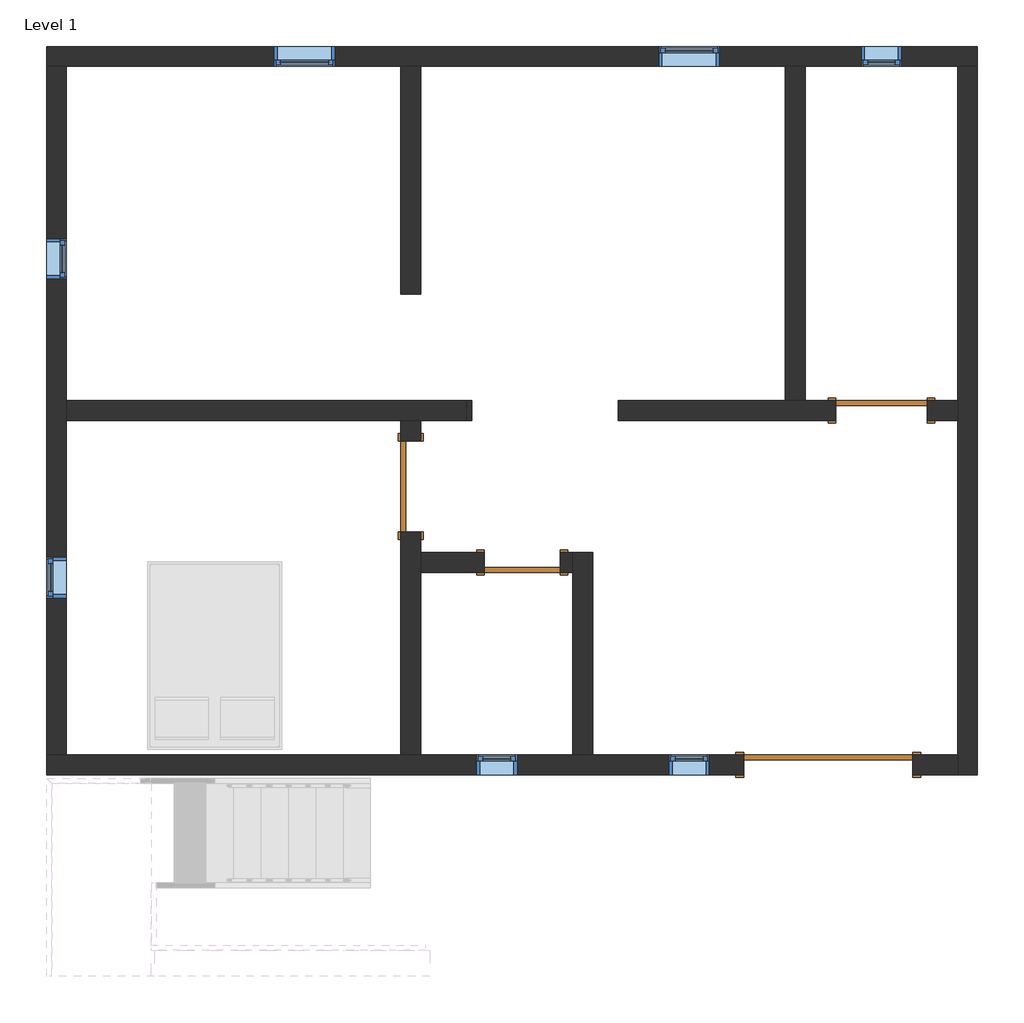
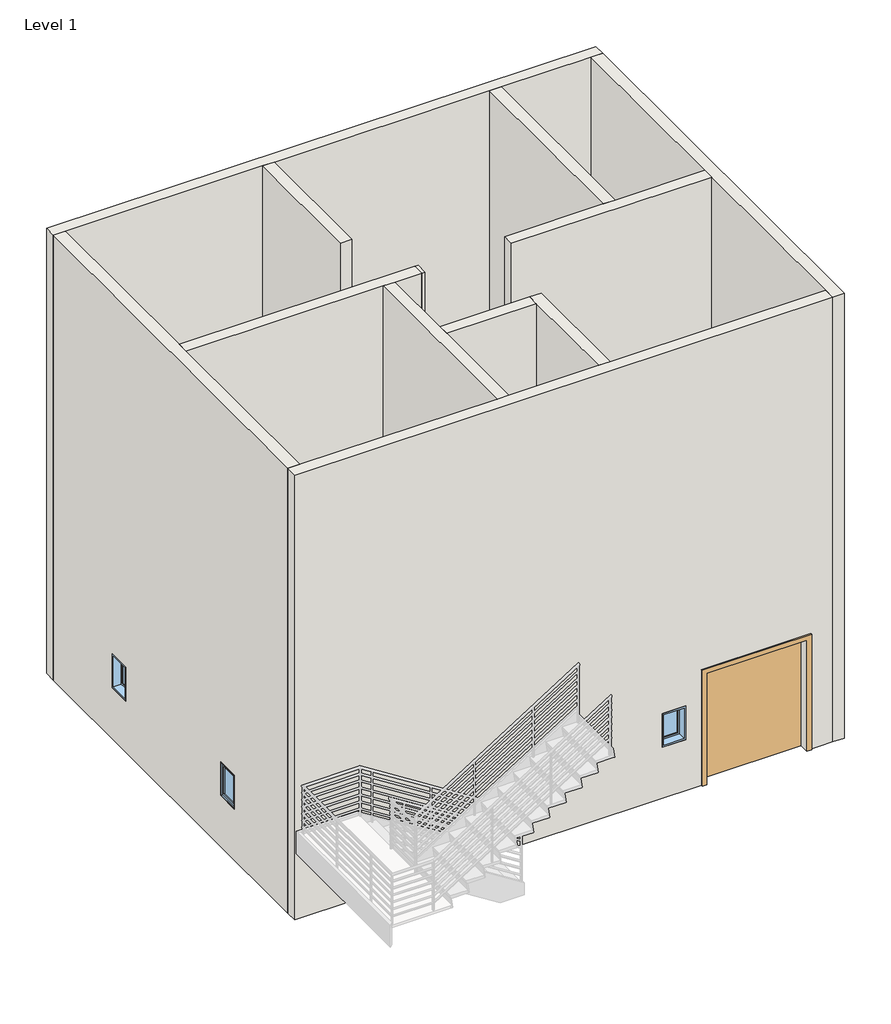
# One storey, part 1 of 4: 12 walls, 7 windows, 4 doors.
"""IFC4 building model written with IfcOpenShell, lengths in millimetres."""

from ifc_helpers import new_model, si_unit, frame, origin, origin_with_axes, place, context, project, spatial, polyline, outline, extrude, faceted_brep, transform, mapped, element, save
from components import m_door_double_flush_panel_double_acting_1700_x_2000mm_0a6d9c7f, m_single_flush_0762_x_2032mm_7341a4fb, m_single_flush_0915_x_2134mm_6a9e8738, m_fixed_0406_x_0610mm_8205b201, m_fixed_0610_x_1220mm_4e981104

model = new_model("IFC4")

# Units and contexts
model_context = context("Model", 3, world=origin())
ifc_project = project(units=[si_unit("LENGTHUNIT", "METRE", prefix="MILLI")], contexts=[model_context])

# Site, building, storey
site = spatial("IfcSite", under=ifc_project)
building = spatial("IfcBuilding", under=site)
storey = spatial("IfcBuildingStorey", under=building, Name="Level 1", Elevation=0.0)

# Doors
placement = place(None, origin())
m_door_double_flush_panel_double_acting_1700_x_2000mm_shape = m_door_double_flush_panel_double_acting_1700_x_2000mm_0a6d9c7f(model_context)
element("IfcDoor", 1, ObjectType="M_Door-Double-Flush_Panel-Double-Acting : 1700 x 2000mm", at=placement, inside=storey, context=model_context, shape_type="MappedRepresentation", body=[
    mapped(m_door_double_flush_panel_double_acting_1700_x_2000mm_shape, transform((-3679.0492596, 6432.7433377, 0.0), x_axis=(1.0, 0.0, 0.0), y_axis=(0.0, 1.0, 0.0), z_axis=(0.0, 0.0, 1.0))),
])
m_single_flush_0762_x_2032mm_shape = m_single_flush_0762_x_2032mm_7341a4fb(model_context)
element("IfcDoor", 2, ObjectType="M_Single-Flush : 0762 x 2032mm", at=placement, inside=storey, context=model_context, shape_type="MappedRepresentation", body=[
    mapped(m_single_flush_0762_x_2032mm_shape, transform((-6752.4492596, 8463.1433377, 0.0), x_axis=(1.0, 0.0, 0.0), y_axis=(0.0, 1.0, 0.0), z_axis=(0.0, 0.0, 1.0))),
])
m_single_flush_0915_x_2134mm_shape = m_single_flush_0915_x_2134mm_6a9e8738(model_context)
element("IfcDoor", 3, ObjectType="M_Single-Flush : 0915 x 2134mm", at=placement, inside=storey, context=model_context, shape_type="MappedRepresentation", body=[
    mapped(m_single_flush_0915_x_2134mm_shape, transform((-3145.6492596, 9988.7433377, 0.0), x_axis=(1.0, 0.0, 0.0), y_axis=(0.0, 1.0, 0.0), z_axis=(0.0, 0.0, 1.0))),
])
element("IfcDoor", 4, ObjectType="M_Single-Flush : 0915 x 2134mm", at=placement, inside=storey, context=model_context, shape_type="MappedRepresentation", body=[
    mapped(m_single_flush_0915_x_2134mm_shape, transform((-7870.0492596, 9226.7433377, 0.0), x_axis=(0.0, 1.0, 0.0), y_axis=(-1.0, 0.0, 0.0), z_axis=(0.0, 0.0, 1.0))),
])

# Walls
element("IfcWall", 5, ObjectType="Generic - 200mm", at=placement, inside=storey, context=model_context, shape_type="Brep", body=[
    faceted_brep([(-11526.0492596, 13444.7433377, 0.0), (-11326.0492596, 13444.7433377, 0.0), (-7970.0492596, 13444.7433377, 0.0), (-7770.0492596, 13444.7433377, 0.0), (-4109.2492596, 13444.7433377, 0.0), (-3909.2492596, 13444.7433377, 0.0), (-2382.0492596, 13444.7433377, 0.0), (-2182.0492596, 13444.7433377, 0.0), (-2182.0492596, 13444.7433377, 8000.0), (-2382.0492596, 13444.7433377, 8000.0), (-3909.2492596, 13444.7433377, 8000.0), (-4109.2492596, 13444.7433377, 8000.0), (-7770.0492596, 13444.7433377, 8000.0), (-7970.0492596, 13444.7433377, 8000.0), (-11326.0492596, 13444.7433377, 8000.0), (-11526.0492596, 13444.7433377, 8000.0), (-8631.8492596, 13444.7433377, 915.0), (-9241.8492596, 13444.7433377, 915.0), (-9241.8492596, 13444.7433377, 2135.0), (-8631.8492596, 13444.7433377, 2135.0), (-5381.0492596, 13444.7433377, 915.0), (-5381.0492596, 13444.7433377, 2135.0), (-4771.0492596, 13444.7433377, 2135.0), (-4771.0492596, 13444.7433377, 915.0), (-2942.6492596, 13444.7433377, 915.0), (-3348.6492596, 13444.7433377, 915.0), (-3348.6492596, 13444.7433377, 1525.0), (-2942.6492596, 13444.7433377, 1525.0), (-11526.0492596, 13644.7433377, 0.0), (-11526.0492596, 13644.7433377, 8000.0), (-2182.0492596, 13644.7433377, 8000.0), (-2182.0492596, 13644.7433377, 0.0), (-8631.8492596, 13644.7433377, 915.0), (-8631.8492596, 13644.7433377, 2135.0), (-9241.8492596, 13644.7433377, 2135.0), (-9241.8492596, 13644.7433377, 915.0), (-5381.0492596, 13644.7433377, 915.0), (-4771.0492596, 13644.7433377, 915.0), (-4771.0492596, 13644.7433377, 2135.0), (-5381.0492596, 13644.7433377, 2135.0), (-2942.6492596, 13644.7433377, 915.0), (-2942.6492596, 13644.7433377, 1525.0), (-3348.6492596, 13644.7433377, 1525.0), (-3348.6492596, 13644.7433377, 915.0)], [[[0, 1, 2, 3, 4, 5, 6, 7, 8, 9, 10, 11, 12, 13, 14, 15], [16, 17, 18, 19], [20, 21, 22, 23], [24, 25, 26, 27]], [[28, 29, 30, 31], [32, 33, 34, 35], [36, 37, 38, 39], [40, 41, 42, 43]], [[7, 6, 5, 4, 3, 2, 1, 0, 28, 31]], [[15, 14, 13, 12, 11, 10, 9, 8, 30, 29]], [[8, 7, 31, 30]], [[0, 15, 29, 28]], [[33, 32, 16, 19]], [[34, 33, 19, 18]], [[35, 34, 18, 17]], [[32, 35, 17, 16]], [[21, 20, 36, 39]], [[22, 21, 39, 38]], [[23, 22, 38, 37]], [[20, 23, 37, 36]], [[41, 40, 24, 27]], [[42, 41, 27, 26]], [[43, 42, 26, 25]], [[40, 43, 25, 24]]]),
])
element("IfcWall", 6, ObjectType="Generic - 200mm", at=placement, inside=storey, context=model_context, shape_type="Brep", body=[
    faceted_brep([(-2382.0492596, 13444.7433377, 0.0), (-2382.0492596, 10088.7433377, 0.0), (-2382.0492596, 9888.7433377, 0.0), (-2382.0492596, 6532.7433377, 0.0), (-2382.0492596, 6332.7433377, 0.0), (-2382.0492596, 6332.7433377, 8000.0), (-2382.0492596, 6532.7433377, 8000.0), (-2382.0492596, 9888.7433377, 8000.0), (-2382.0492596, 10088.7433377, 8000.0), (-2382.0492596, 13444.7433377, 8000.0), (-2182.0492596, 13444.7433377, 0.0), (-2182.0492596, 13444.7433377, 8000.0), (-2182.0492596, 6332.7433377, 8000.0), (-2182.0492596, 6332.7433377, 0.0)], [[[0, 1, 2, 3, 4, 5, 6, 7, 8, 9]], [[10, 11, 12, 13]], [[4, 3, 2, 1, 0, 10, 13]], [[9, 8, 7, 6, 5, 12, 11]], [[0, 9, 11, 10]], [[5, 4, 13, 12]]]),
])
element("IfcWall", 7, ObjectType="Generic - 200mm", at=placement, inside=storey, context=model_context, shape_type="Brep", body=[
    faceted_brep([(-11526.0492596, 6532.7433377, 8000.0), (-11326.0492596, 6532.7433377, 8000.0), (-7970.0492596, 6532.7433377, 8000.0), (-7770.0492596, 6532.7433377, 8000.0), (-6242.8492596, 6532.7433377, 8000.0), (-6042.8492596, 6532.7433377, 8000.0), (-2382.0492596, 6532.7433377, 8000.0), (-2382.0492596, 6532.7433377, 0.0), (-2829.0492596, 6532.7433377, 0.0), (-2829.0492596, 6532.7433377, 2000.0), (-4529.0492596, 6532.7433377, 2000.0), (-4529.0492596, 6532.7433377, 0.0), (-6042.8492596, 6532.7433377, 0.0), (-6242.8492596, 6532.7433377, 0.0), (-7770.0492596, 6532.7433377, 0.0), (-7970.0492596, 6532.7433377, 0.0), (-11326.0492596, 6532.7433377, 0.0), (-11526.0492596, 6532.7433377, 0.0), (-7209.4492596, 6532.7433377, 915.0), (-6803.4492596, 6532.7433377, 915.0), (-6803.4492596, 6532.7433377, 1525.0), (-7209.4492596, 6532.7433377, 1525.0), (-5279.0492596, 6532.7433377, 915.0), (-4873.0492596, 6532.7433377, 915.0), (-4873.0492596, 6532.7433377, 1525.0), (-5279.0492596, 6532.7433377, 1525.0), (-2382.0492596, 6332.7433377, 8000.0), (-11526.0492596, 6332.7433377, 8000.0), (-11526.0492596, 6332.7433377, 0.0), (-4529.0492596, 6332.7433377, 0.0), (-4529.0492596, 6332.7433377, 2000.0), (-2829.0492596, 6332.7433377, 2000.0), (-2829.0492596, 6332.7433377, 0.0), (-2382.0492596, 6332.7433377, 0.0), (-7209.4492596, 6332.7433377, 915.0), (-7209.4492596, 6332.7433377, 1525.0), (-6803.4492596, 6332.7433377, 1525.0), (-6803.4492596, 6332.7433377, 915.0), (-5279.0492596, 6332.7433377, 915.0), (-5279.0492596, 6332.7433377, 1525.0), (-4873.0492596, 6332.7433377, 1525.0), (-4873.0492596, 6332.7433377, 915.0)], [[[0, 1, 2, 3, 4, 5, 6, 7, 8, 9, 10, 11, 12, 13, 14, 15, 16, 17], [18, 19, 20, 21], [22, 23, 24, 25]], [[26, 27, 28, 29, 30, 31, 32, 33], [34, 35, 36, 37], [38, 39, 40, 41]], [[7, 33, 32, 8]], [[28, 17, 16, 15, 14, 13, 12, 11, 29]], [[6, 5, 4, 3, 2, 1, 0, 27, 26]], [[7, 6, 26, 33]], [[0, 17, 28, 27]], [[35, 34, 18, 21]], [[36, 35, 21, 20]], [[37, 36, 20, 19]], [[34, 37, 19, 18]], [[39, 38, 22, 25]], [[40, 39, 25, 24]], [[41, 40, 24, 23]], [[38, 41, 23, 22]], [[31, 9, 8, 32]], [[9, 31, 30, 10]], [[10, 30, 29, 11]]]),
])
element("IfcWall", 8, ObjectType="Generic - 200mm", at=placement, inside=storey, context=model_context, shape_type="Brep", body=[
    faceted_brep([(-11326.0492596, 6532.7433377, 0.0), (-11326.0492596, 9888.7433377, 0.0), (-11326.0492596, 10088.7433377, 0.0), (-11326.0492596, 13444.7433377, 0.0), (-11326.0492596, 13444.7433377, 8000.0), (-11326.0492596, 10088.7433377, 8000.0), (-11326.0492596, 9888.7433377, 8000.0), (-11326.0492596, 6532.7433377, 8000.0), (-11326.0492596, 11715.7433377, 915.0), (-11326.0492596, 11309.7433377, 915.0), (-11326.0492596, 11309.7433377, 1525.0), (-11326.0492596, 11715.7433377, 1525.0), (-11326.0492596, 8109.3433377, 915.0), (-11326.0492596, 8109.3433377, 1525.0), (-11326.0492596, 8515.3433377, 1525.0), (-11326.0492596, 8515.3433377, 915.0), (-11526.0492596, 6532.7433377, 0.0), (-11526.0492596, 6532.7433377, 8000.0), (-11526.0492596, 13444.7433377, 8000.0), (-11526.0492596, 13444.7433377, 0.0), (-11526.0492596, 11715.7433377, 915.0), (-11526.0492596, 11715.7433377, 1525.0), (-11526.0492596, 11309.7433377, 1525.0), (-11526.0492596, 11309.7433377, 915.0), (-11526.0492596, 8109.3433377, 915.0), (-11526.0492596, 8515.3433377, 915.0), (-11526.0492596, 8515.3433377, 1525.0), (-11526.0492596, 8109.3433377, 1525.0)], [[[0, 1, 2, 3, 4, 5, 6, 7], [8, 9, 10, 11], [12, 13, 14, 15]], [[16, 17, 18, 19], [20, 21, 22, 23], [24, 25, 26, 27]], [[3, 2, 1, 0, 16, 19]], [[7, 6, 5, 4, 18, 17]], [[4, 3, 19, 18]], [[0, 7, 17, 16]], [[21, 20, 8, 11]], [[22, 21, 11, 10]], [[23, 22, 10, 9]], [[20, 23, 9, 8]], [[13, 12, 24, 27]], [[14, 13, 27, 26]], [[15, 14, 26, 25]], [[12, 15, 25, 24]]]),
])
element("IfcWall", 9, ObjectType="Generic - 200mm", at=placement, inside=storey, context=model_context, shape_type="Brep", body=[
    faceted_brep([(-11326.0492596, 9888.7433377, 0.0), (-7970.0492596, 9888.7433377, 0.0), (-7770.0492596, 9888.7433377, 0.0), (-7314.3677357, 9888.7433377, 0.0), (-7314.3677357, 9888.7433377, 8000.0), (-7770.0492596, 9888.7433377, 8000.0), (-7970.0492596, 9888.7433377, 8000.0), (-11326.0492596, 9888.7433377, 8000.0), (-11326.0492596, 10088.7433377, 0.0), (-11326.0492596, 10088.7433377, 8000.0), (-7314.3677357, 10088.7433377, 8000.0), (-7314.3677357, 10088.7433377, 0.0)], [[[0, 1, 2, 3, 4, 5, 6, 7]], [[8, 9, 10, 11]], [[3, 2, 1, 0, 8, 11]], [[4, 3, 11, 10]], [[7, 6, 5, 4, 10, 9]], [[0, 7, 9, 8]]]),
])
element("IfcWall", 10, ObjectType="Generic - 200mm", at=placement, inside=storey, context=model_context, shape_type="SweptSolid", body=[
    extrude(outline(polyline([(-4109.2492596, 10088.7433377), (-4109.2492596, 13444.7433377), (-3909.2492596, 13444.7433377), (-3909.2492596, 10088.7433377), (-4109.2492596, 10088.7433377)])), origin_with_axes(), (0.0, 0.0, 1.0), 8000.0),
])
element("IfcWall", 11, ObjectType="Generic - 200mm", at=placement, inside=storey, context=model_context, shape_type="Brep", body=[
    faceted_brep([(-2382.0492596, 10088.7433377, 0.0), (-2688.1492596, 10088.7433377, 0.0), (-2688.1492596, 10088.7433377, 2134.0), (-3603.1492596, 10088.7433377, 2134.0), (-3603.1492596, 10088.7433377, 0.0), (-3909.2492596, 10088.7433377, 0.0), (-4109.2492596, 10088.7433377, 0.0), (-5787.2492596, 10088.7433377, 0.0), (-5787.2492596, 10088.7433377, 8000.0), (-4109.2492596, 10088.7433377, 8000.0), (-3909.2492596, 10088.7433377, 8000.0), (-2382.0492596, 10088.7433377, 8000.0), (-2688.1492596, 9888.7433377, 2134.0), (-2688.1492596, 9888.7433377, 0.0), (-2382.0492596, 9888.7433377, 0.0), (-2382.0492596, 9888.7433377, 8000.0), (-5787.2492596, 9888.7433377, 8000.0), (-5787.2492596, 9888.7433377, 0.0), (-3603.1492596, 9888.7433377, 0.0), (-3603.1492596, 9888.7433377, 2134.0)], [[[0, 1, 2, 3, 4, 5, 6, 7, 8, 9, 10, 11]], [[12, 13, 14, 15, 16, 17, 18, 19]], [[18, 17, 7, 6, 5, 4]], [[14, 13, 1, 0]], [[8, 7, 17, 16]], [[11, 10, 9, 8, 16, 15]], [[0, 11, 15, 14]], [[2, 1, 13, 12]], [[3, 2, 12, 19]], [[4, 3, 19, 18]]]),
])
element("IfcWall", 12, ObjectType="Generic - 200mm", at=placement, inside=storey, context=model_context, shape_type="SweptSolid", body=[
    extrude(outline(polyline([(-7260.4492596, 9888.7433377), (-7314.3677357, 9888.7433377), (-7314.3677357, 10088.7433377), (-7260.4492596, 10088.7433377), (-7260.4492596, 9888.7433377)])), origin_with_axes(), (0.0, 0.0, 1.0), 8000.0),
])
element("IfcWall", 13, ObjectType="Generic - 200mm", at=placement, inside=storey, context=model_context, shape_type="SweptSolid", body=[
    extrude(outline(polyline([(-7970.0492596, 11158.7433377), (-7970.0492596, 13444.7433377), (-7770.0492596, 13444.7433377), (-7770.0492596, 11158.7433377), (-7970.0492596, 11158.7433377)])), origin_with_axes(), (0.0, 0.0, 1.0), 8000.0),
])
element("IfcWall", 14, ObjectType="Generic - 200mm", at=placement, inside=storey, context=model_context, shape_type="Brep", body=[
    faceted_brep([(-7770.0492596, 9684.2433377, 2134.0), (-7770.0492596, 9684.2433377, 0.0), (-7770.0492596, 9888.7433377, 0.0), (-7770.0492596, 9888.7433377, 8000.0), (-7770.0492596, 8563.1433377, 8000.0), (-7770.0492596, 8363.1433377, 8000.0), (-7770.0492596, 6532.7433377, 8000.0), (-7770.0492596, 6532.7433377, 0.0), (-7770.0492596, 8363.1433377, 0.0), (-7770.0492596, 8563.1433377, 0.0), (-7770.0492596, 8769.2433377, 0.0), (-7770.0492596, 8769.2433377, 2134.0), (-7970.0492596, 9888.7433377, 0.0), (-7970.0492596, 9684.2433377, 0.0), (-7970.0492596, 9684.2433377, 2134.0), (-7970.0492596, 8769.2433377, 2134.0), (-7970.0492596, 8769.2433377, 0.0), (-7970.0492596, 6532.7433377, 0.0), (-7970.0492596, 6532.7433377, 8000.0), (-7970.0492596, 9888.7433377, 8000.0)], [[[0, 1, 2, 3, 4, 5, 6, 7, 8, 9, 10, 11]], [[12, 13, 14, 15, 16, 17, 18, 19]], [[2, 1, 13, 12]], [[10, 9, 8, 7, 17, 16]], [[6, 5, 4, 3, 19, 18]], [[7, 6, 18, 17]], [[3, 2, 12, 19]], [[14, 13, 1, 0]], [[15, 14, 0, 11]], [[16, 15, 11, 10]]]),
])
element("IfcWall", 15, ObjectType="Generic - 200mm", at=placement, inside=storey, context=model_context, shape_type="Brep", body=[
    faceted_brep([(-6042.8492596, 6532.7433377, 0.0), (-6042.8492596, 8563.1433377, 0.0), (-6042.8492596, 8563.1433377, 8000.0), (-6042.8492596, 6532.7433377, 8000.0), (-6242.8492596, 6532.7433377, 0.0), (-6242.8492596, 6532.7433377, 8000.0), (-6242.8492596, 8363.1433377, 8000.0), (-6242.8492596, 8563.1433377, 8000.0), (-6242.8492596, 8563.1433377, 0.0), (-6242.8492596, 8363.1433377, 0.0)], [[[0, 1, 2, 3]], [[4, 5, 6, 7, 8, 9]], [[1, 0, 4, 9, 8]], [[3, 2, 7, 6, 5]], [[0, 3, 5, 4]], [[2, 1, 8, 7]]]),
])
element("IfcWall", 16, ObjectType="Generic - 200mm", at=placement, inside=storey, context=model_context, shape_type="SweptSolid", body=[
    extrude(outline(polyline([(2032.0, -6371.4492596), (0.0, -6371.4492596), (0.0, -6242.8492596), (8000.0, -6242.8492596), (8000.0, -7770.0492596), (0.0, -7770.0492596), (0.0, -7133.4492596), (2032.0, -7133.4492596), (2032.0, -6371.4492596)])), frame((0.0, 8363.1433377, 0.0), z_axis=(0.0, 1.0, 0.0), x_axis=(0.0, 0.0, 1.0)), (0.0, 0.0, 1.0), 200.0),
])

# Windows
m_fixed_0406_x_0610mm_shape = m_fixed_0406_x_0610mm_8205b201(model_context)
element("IfcWindow", 17, ObjectType="M_Fixed : 0406 x 0610mm", at=placement, inside=storey, context=model_context, shape_type="MappedRepresentation", body=[
    mapped(m_fixed_0406_x_0610mm_shape, transform((-3145.6492596, 13557.7433377, 0.0), x_axis=(-1.0, 0.0, 0.0), y_axis=(0.0, -1.0, 0.0), z_axis=(0.0, 0.0, 1.0))),
])
element("IfcWindow", 18, ObjectType="M_Fixed : 0406 x 0610mm", at=placement, inside=storey, context=model_context, shape_type="MappedRepresentation", body=[
    mapped(m_fixed_0406_x_0610mm_shape, transform((-7006.4492596, 6419.7433377, 0.0), x_axis=(1.0, 0.0, 0.0), y_axis=(0.0, 1.0, 0.0), z_axis=(0.0, 0.0, 1.0))),
])
element("IfcWindow", 19, ObjectType="M_Fixed : 0406 x 0610mm", at=placement, inside=storey, context=model_context, shape_type="MappedRepresentation", body=[
    mapped(m_fixed_0406_x_0610mm_shape, transform((-11439.0492596, 11512.7433377, 0.0), x_axis=(0.0, -1.0, 0.0), y_axis=(1.0, 0.0, 0.0), z_axis=(0.0, 0.0, 1.0))),
])
element("IfcWindow", 20, ObjectType="M_Fixed : 0406 x 0610mm", at=placement, inside=storey, context=model_context, shape_type="MappedRepresentation", body=[
    mapped(m_fixed_0406_x_0610mm_shape, transform((-11413.0492596, 8312.3433377, 0.0), x_axis=(0.0, 1.0, 0.0), y_axis=(-1.0, 0.0, 0.0), z_axis=(0.0, 0.0, 1.0))),
])
element("IfcWindow", 21, ObjectType="M_Fixed : 0406 x 0610mm", at=placement, inside=storey, context=model_context, shape_type="MappedRepresentation", body=[
    mapped(m_fixed_0406_x_0610mm_shape, transform((-5076.0492596, 6419.7433377, 0.0), x_axis=(1.0, 0.0, 0.0), y_axis=(0.0, 1.0, 0.0), z_axis=(0.0, 0.0, 1.0))),
])
m_fixed_0610_x_1220mm_shape = m_fixed_0610_x_1220mm_4e981104(model_context)
element("IfcWindow", 22, ObjectType="M_Fixed : 0610 x 1220mm", at=placement, inside=storey, context=model_context, shape_type="MappedRepresentation", body=[
    mapped(m_fixed_0610_x_1220mm_shape, transform((-8936.8492596, 13557.7433377, 0.0), x_axis=(-1.0, 0.0, 0.0), y_axis=(0.0, -1.0, 0.0), z_axis=(0.0, 0.0, 1.0))),
])
element("IfcWindow", 23, ObjectType="M_Fixed : 0610 x 1220mm", at=placement, inside=storey, context=model_context, shape_type="MappedRepresentation", body=[
    mapped(m_fixed_0610_x_1220mm_shape, transform((-5076.0492596, 13531.7433377, 0.0), x_axis=(1.0, 0.0, 0.0), y_axis=(0.0, 1.0, 0.0), z_axis=(0.0, 0.0, 1.0))),
])

save(model, "model.ifc")

# Revit data of these elements
# Type "M_Door-Double-Flush_Panel-Double-Acting : 1700 x 2000mm"
#   Type Mark = "22"
#   Construction Type Id = "DOOR"
#   Assembly Code = "C1020"
#   Analytic Construction = "Wooden"
#   W = 850 mm
#   Thickness = 50 mm
#   Thermal Resistance (R) = 0.455703 (m²·K)/W
#   Swing Angle [instance default] = 90.00°
#   Heat Transfer Coefficient (U) = 2.19465 W/(m²·K)
#   Height = 2000 mm
#   Trim Projection Ext. = 25 mm
#   Trim Projection Int. = 25 mm
#   Trim Width Ext. = 80 mm
#   Trim Width Int. = 80 mm
#   Width = 1700 mm
#   Define Thermal Properties by = 1
#   Panel Material = Wood - Birch - Solid Stained Light Low Gloss
#   Trim Material = Paint - Sienna
#   Visual Light Transmittance = 0
#   Solar Heat Gain Coefficient = 0
#   Function = (empty or 0)
#   Wall Closure = (empty or 0)
# Type "M_Single-Flush : 0762 x 2032mm"
#   Type Mark = "19"
#   Thickness = 51 mm
#   Height = 2032 mm
#   Trim Projection Ext = 25 mm
#   Trim Projection Int = 25 mm
#   Trim Width = 76 mm
#   Width = 762 mm
#   Door Material = Door - Panel
#   Frame Material = Door - Frame
#   Function = (empty or 0)
#   Wall Closure = (empty or 0)
# Type "M_Single-Flush : 0915 x 2134mm"
#   Type Mark = "15"
#   Thickness = 51 mm
#   Height = 2134 mm
#   Trim Projection Ext = 25 mm
#   Trim Projection Int = 25 mm
#   Trim Width = 76 mm
#   Width = 915 mm
#   Door Material = Door - Panel
#   Frame Material = Door - Frame
#   Function = (empty or 0)
#   Wall Closure = (empty or 0)
# Type "Generic - 200mm"
#   Layers, outside or top first: 200 mm no material (function 1)
# Type "M_Fixed : 0406 x 0610mm"
#   Type Mark = "10"
#   Height = 610 mm
#   Default Sill Height = 915 mm
#   Width = 406 mm
#   Window Inset = 19 mm
#   Frame Exterior Material = Sash
#   Frame Interior Material = Sash
#   Glass Pane Material = Glass
#   Sash = Sash
#   Wall Closure = (empty or 0)
# Type "M_Fixed : 0610 x 1220mm"
#   Type Mark = "13"
#   Height = 1220 mm
#   Default Sill Height = 915 mm
#   Width = 610 mm
#   Window Inset = 19 mm
#   Frame Exterior Material = Sash
#   Frame Interior Material = Sash
#   Glass Pane Material = Glass
#   Sash = Sash
#   Wall Closure = (empty or 0)
# Element 1 (IfcDoor, "M_Door-Double-Flush_Panel-Double-Acting : 1700 x 2000mm")
#   Swing Angle = 90.00°
#   Phase Created = New Construction
#   Materials on its faces: "Paint - Sienna", "Wood - Birch - Solid Stained Light Low Gloss"
# Element 2 (IfcDoor, "M_Single-Flush : 0762 x 2032mm")
#   Phase Created = New Construction
#   Materials on its faces: "Door - Frame", "Door - Panel"
# Elements 3, 4 (IfcDoor, "M_Single-Flush : 0915 x 2134mm")
#   Phase Created = New Construction
#   Materials on its faces: "Door - Frame", "Door - Panel"
# Elements 5, 6, 7, 8, 9, 10, 11, 12, 13, 14, 15, 16 (IfcWall, "Generic - 200mm")
#   Top Offset = 0 mm
#   Base Offset = 0 mm
#   Unconnected Height = 8000 mm
#   wall height = 8000 mm
#   Phase Created = New Construction
#   Base Constraint = Level 1
#   Materials on its faces: "Default Wall"
# Element 17 (IfcWindow, "M_Fixed : 0406 x 0610mm")
#   Mark = "8"
#   Phase Created = New Construction
#   Materials on its faces: "Sash", "Glass"
# Element 18 (IfcWindow, "M_Fixed : 0406 x 0610mm")
#   Mark = "9"
#   Phase Created = New Construction
#   Materials on its faces: "Sash", "Glass"
# Element 19 (IfcWindow, "M_Fixed : 0406 x 0610mm")
#   Mark = "10"
#   Phase Created = New Construction
#   Materials on its faces: "Sash", "Glass"
# Element 20 (IfcWindow, "M_Fixed : 0406 x 0610mm")
#   Mark = "11"
#   Phase Created = New Construction
#   Materials on its faces: "Sash", "Glass"
# Element 21 (IfcWindow, "M_Fixed : 0406 x 0610mm")
#   Mark = "12"
#   Phase Created = New Construction
#   Materials on its faces: "Sash", "Glass"
# Element 22 (IfcWindow, "M_Fixed : 0610 x 1220mm")
#   Mark = "6"
#   Phase Created = New Construction
#   Materials on its faces: "Sash", "Glass"
# Element 23 (IfcWindow, "M_Fixed : 0610 x 1220mm")
#   Mark = "7"
#   Phase Created = New Construction
#   Materials on its faces: "Sash", "Glass"
# Materials
#   "Wood - Birch - Solid Stained Light Low Gloss": class "Wood", colour RGB 210 159 95, transparency 0, Cost = 0
#   "Paint - Sienna": colour RGB 118 70 51, transparency 0, Cost = 0
#   "Door - Panel": class "Wood", colour RGB 114 82 51, transparency 0
#   "Door - Frame": colour RGB 153 76 43, transparency 0
#   "Sash": class "Wood", colour RGB 136 99 55, transparency 0
#   "Glass": class "Glass", colour RGB 218 227 224, transparency 0.85, Description = "Soda Lime Glass", Cost = 0
#   "Default Wall": colour RGB 80 80 80, transparency 0
